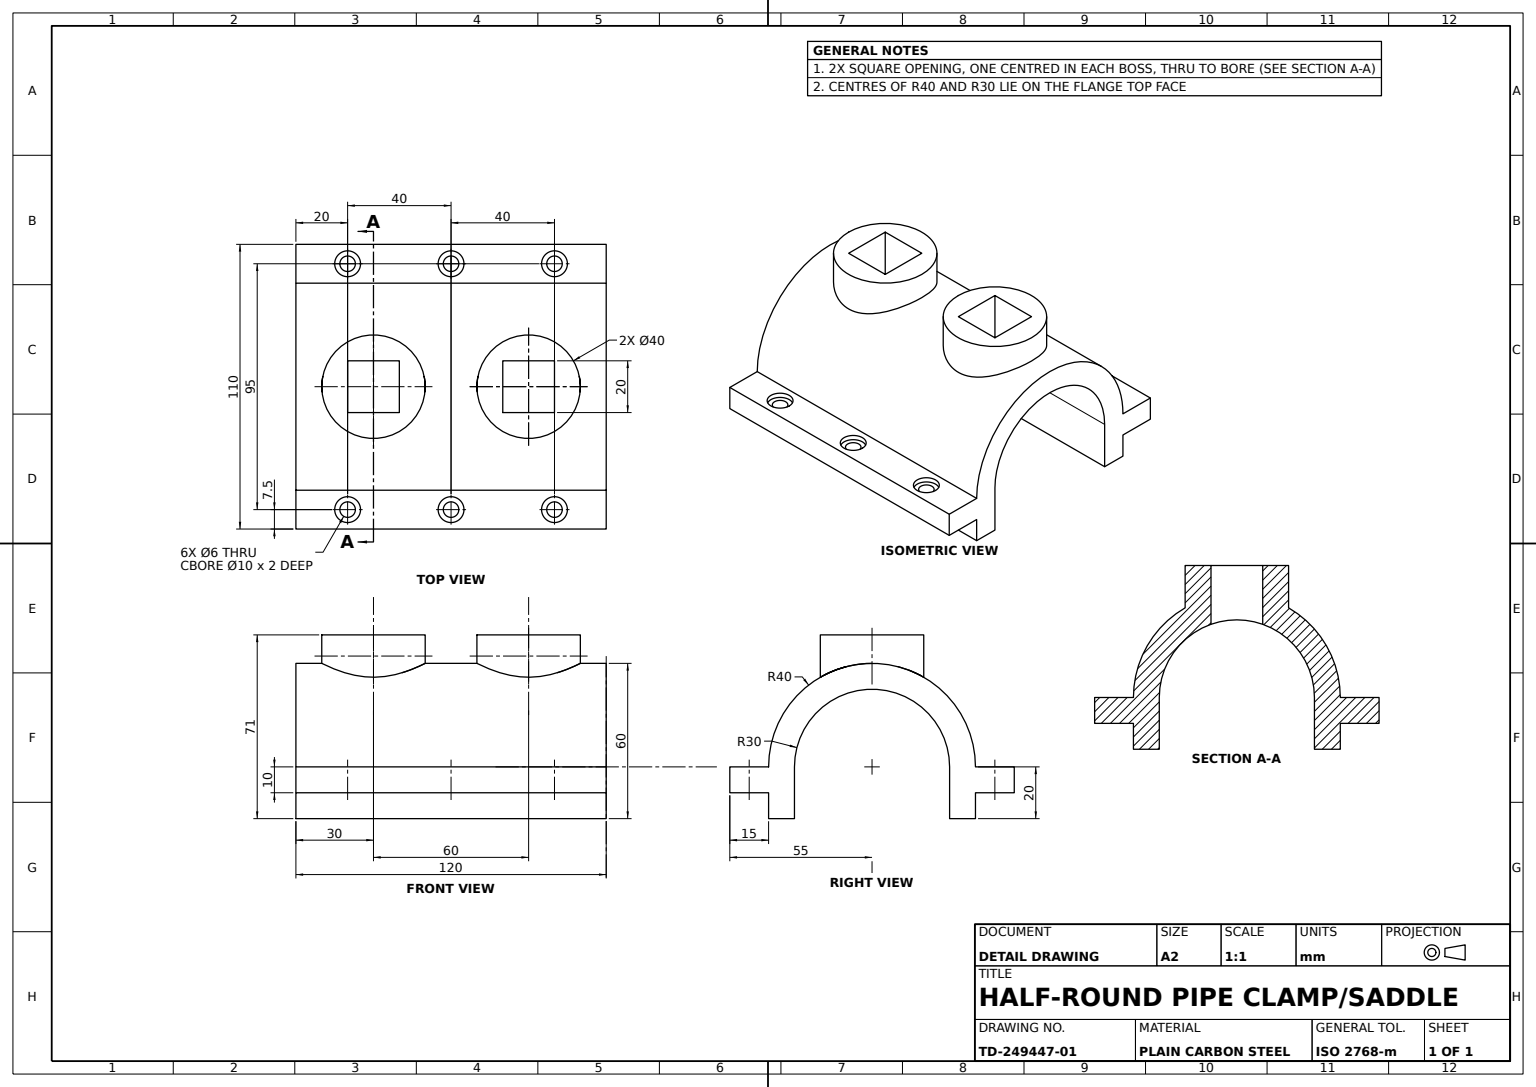
SolidWorks part; units mm, degrees
material "Plain Carbon Steel"
ref_plane "Front Plane" through (0, 0, 0) normal (0, 0, 1) x (1, 0, 0)
ref_plane "Top Plane" through (0, 0, 0) normal (0, 1, 0) x (1, 0, 0)
ref_plane "Right Plane" through (0, 0, 0) normal (1, 0, 0) x (0, 0, -1)
sketch "Cap Profile Sketch" plane through (0, 0, 0) normal (0, 0, 1) x (1, 0, 0)
  line L2 (-55, 0) -> (-40, 0)
  line L3 (-30, 0) -> (-30, -20)
  line L4 (-30, -20) -> (-40, -20)
  line L5 (-40, -20) -> (-40, -10)
  line L6 (-40, -10) -> (-55, -10)
  line L7 (-55, -10) -> (-55, 0)
  line L8 (30, 0) -> (30, -20)
  line L9 (30, -20) -> (40, -20)
  line L10 (40, -20) -> (40, -10)
  line L11 (40, -10) -> (55, -10)
  line L12 (55, -10) -> (55, 0)
  line L13 (40, 0) -> (55, 0)
  arc A0 (30, 0) -> (-30, 0) centre (0, 0) ccw
  arc A1 (40, 0) -> (-40, 0) centre (0, 0) ccw
  point P8 (0, 0)
  dimension "D1" = 80
  dimension "D2" = 60
  dimension "D3" = 15
  dimension "D4" = 15
  dimension "D5" = 10
  dimension "D6" = 10
  dimension "D7" = 55
  dimension "D8" = 80
  dimension "D9" = 10
  dimension "D10" = 20
extrude "Half Pipe Cap Body" add sketch "Cap Profile Sketch" along normal blind 120
sketch "Mounting Holes Sketch" plane through (0, 0, 0) normal (0, 1, 0) x (1, 0, 0)
  line L0 (-40, 0) -> (-55, 0) construction
  line L1 (-40, -120) -> (-55, -120) construction
  circle A0 centre (-47.5, -20) radius 3
  circle A2 centre (-47.5, -100) radius 3
  circle A3 centre (-47.5, -60) radius 3
  circle A4 centre (47.5, -20) radius 3
  circle A5 centre (47.5, -60) radius 3
  circle A6 centre (47.5, -100) radius 3
  dimension "D1" = 6
  dimension "D2" = 6
  dimension "D3" = 6
  dimension "D5" = 6
  dimension "D6" = 6
  dimension "D7" = 6
  dimension "D4" = 20
  dimension "D8" = 95
  dimension "D9" = 95
  dimension "D10" = 20
  dimension "D11" = 40
  dimension "D12" = 40
  dimension "D13" = 40
  dimension "D14" = 40
  dimension "D15" = 47.5
  dimension "D16" = 100
extrude "Mounting Holes 6xØ6" cut sketch "Mounting Holes Sketch" against normal blind 120
sketch "Counterbore Sketch" plane through (0, 0, 0) normal (0, 1, 0) x (1, 0, 0)
  circle A0 centre (-47.5, -20) radius 5
  circle A1 centre (-47.5, -60) radius 5
  circle A2 centre (-47.5, -100) radius 5
  circle A3 centre (47.5, -100) radius 5
  circle A4 centre (47.5, -60) radius 5
  circle A5 centre (47.5, -20) radius 5
  circle A6 centre (-47.5, -20) radius 0.003
  circle A7 centre (-47.5, -60) radius 3
  circle A8 centre (-47.5, -100) radius 3
  circle A9 centre (-47.5, -20) radius 3
  circle A10 centre (47.5, -20) radius 3
  circle A11 centre (47.5, -60) radius 3
  circle A12 centre (47.5, -100) radius 3
  circle M1 centre (-47.5, -60) radius 3
  circle M2 centre (-47.5, -100) radius 3
  circle M3 centre (-47.5, -20) radius 3
  dimension "D1" = 10
  dimension "D2" = 10
  dimension "D3" = 10
  dimension "D4" = 10
  dimension "D5" = 10
  dimension "D6" = 10
  dimension "D7" = 6
  dimension "D8" = 6
  dimension "D9" = 6
  dimension "D10" = 6
  dimension "D11" = 6
  dimension "D12" = 6
  dimension "D13" = 0.006
extrude "Counterbores 6xØ10x2" cut sketch "Counterbore Sketch" against normal blind 2 contours A1 M1 | A2 M2 | A0 M3 | A5 A10 | A4 A11 | A3 A12
ref_plane "Boss Sketch Plane" through (0, 31, 0) normal (0, 1, 0) x (1, 0, 0)
sketch "Boss Sketch" plane through (0, 31, 0) normal (0, 1, 0) x (1, 0, 0)
  line L0 (-40, -120) -> (40, -120) construction
  line L2 (-10, -40) -> (10, -40)
  line L3 (-10, -40) -> (-10, -20)
  line L4 (-10, -20) -> (10, -20)
  line L5 (10, -40) -> (10, -20)
  line L6 (-10, -40) -> (10, -20) construction
  line L7 (-10, -20) -> (10, -40) construction
  line L8 (-10, -100) -> (10, -100)
  line L9 (-10, -100) -> (-10, -80)
  line L10 (-10, -80) -> (10, -80)
  line L11 (10, -100) -> (10, -80)
  line L12 (-10, -100) -> (10, -80) construction
  line L13 (-10, -80) -> (10, -100) construction
  circle A0 centre (0, -30) radius 20
  circle A1 centre (0, -90) radius 20
  dimension "D1" = 40
  dimension "D2" = 40
  dimension "D3" = 60
  dimension "D4" = 30
  dimension "D5" = 30
  dimension "D6" = 20
  dimension "D7" = 20
extrude "Top Bosses 2xØ40" add sketch "Boss Sketch" along normal blind 20
sketch "Square Socket Sketch" plane through (0, 31, 0) normal (0, 1, 0) x (1, 0, 0)
  line L1 (-10, -20) -> (10, -20)
  line L2 (-10, -20) -> (-10, -40)
  line L3 (-10, -40) -> (10, -40)
  line L4 (10, -20) -> (10, -40)
  line L5 (-10, -20) -> (10, -40) construction
  line L6 (-10, -40) -> (10, -20) construction
  line L7 (-10, -80) -> (10, -80)
  line L8 (-10, -80) -> (-10, -100)
  line L9 (-10, -100) -> (10, -100)
  line L10 (10, -80) -> (10, -100)
  line L11 (-10, -80) -> (10, -100) construction
  line L12 (-10, -100) -> (10, -80) construction
  point P0 (0, -30)
  point P5 (0, -90)
  dimension "D1" = 20
  dimension "D2" = 20
extrude "Square Sockets 2x20x20" cut sketch "Square Socket Sketch" against normal mid plane 40
